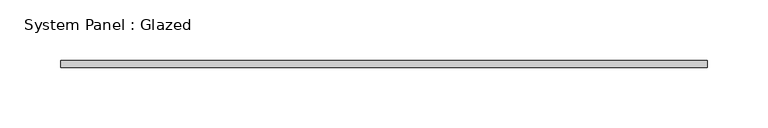
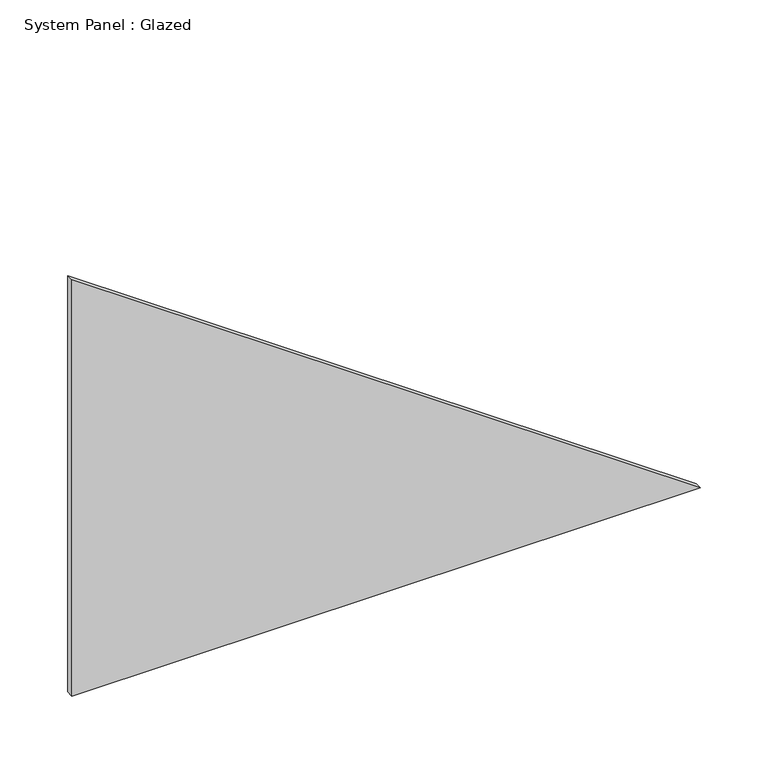
"""IFC4 building model written with IfcOpenShell, lengths in millimetres: plate geometry, System Panel : Glazed."""

from ifc_helpers import new_model, si_unit, frame, origin, place, context, project, spatial, polyline, outline, extrude, source, transform, mapped, element, save


def system_panel_glazed_9e355314(model_context):
    return source(origin(), model_context, "Body", "SweptSolid", [
        extrude(outline(polyline([(0.0, -267.2657279), (0.0, 267.2657279), (374.2829548, -267.2657279), (0.0, -267.2657279)])), frame((0.0, 34.0, 0.0), z_axis=(0.0, 1.0, 0.0), x_axis=(0.0, 0.0, 1.0)), (0.0, 0.0, 1.0), 6.0),
    ])


if __name__ == "__main__":
    model = new_model("IFC4")
    model_context = context("Model", 3, world=origin())
    ifc_project = project(units=[si_unit("LENGTHUNIT", "METRE", prefix="MILLI")], contexts=[model_context])
    site = spatial("IfcSite", under=ifc_project)
    building = spatial("IfcBuilding", under=site)
    placement = place(None, origin())
    system_panel_glazed_shape = system_panel_glazed_9e355314(model_context)
    element("IfcPlate", 1, ObjectType="System Panel : Glazed", at=placement, inside=building, context=model_context, shape_type="MappedRepresentation", body=[
        mapped(system_panel_glazed_shape, transform((0.0, 0.0, 0.0), x_axis=(1.0, 0.0, 0.0), y_axis=(0.0, 1.0, 0.0), z_axis=(0.0, 0.0, 1.0))),
    ])
    save(model, "model.ifc")

# Revit data of these elements
# Type "System Panel : Glazed"
#   Construction Type Id = "GSP4R"
#   Analytic Construction = "1/8 in Pilkington single glazing"
#   Visual Light Transmittance = 0.9
#   Solar Heat Gain Coefficient = 0.86
#   Heat Transfer Coefficient (U) = 6.7069 W/(m²·K)
#   Define Thermal Properties by = 1
# Element 1 (IfcPlate, "System Panel : Glazed")
#   Materials on its faces: "Default New Material(6)"
# Materials
#   "Default New Material(6)": class "Generic", colour RGB 191 25 25, transparency 0.9, Cost = 0
